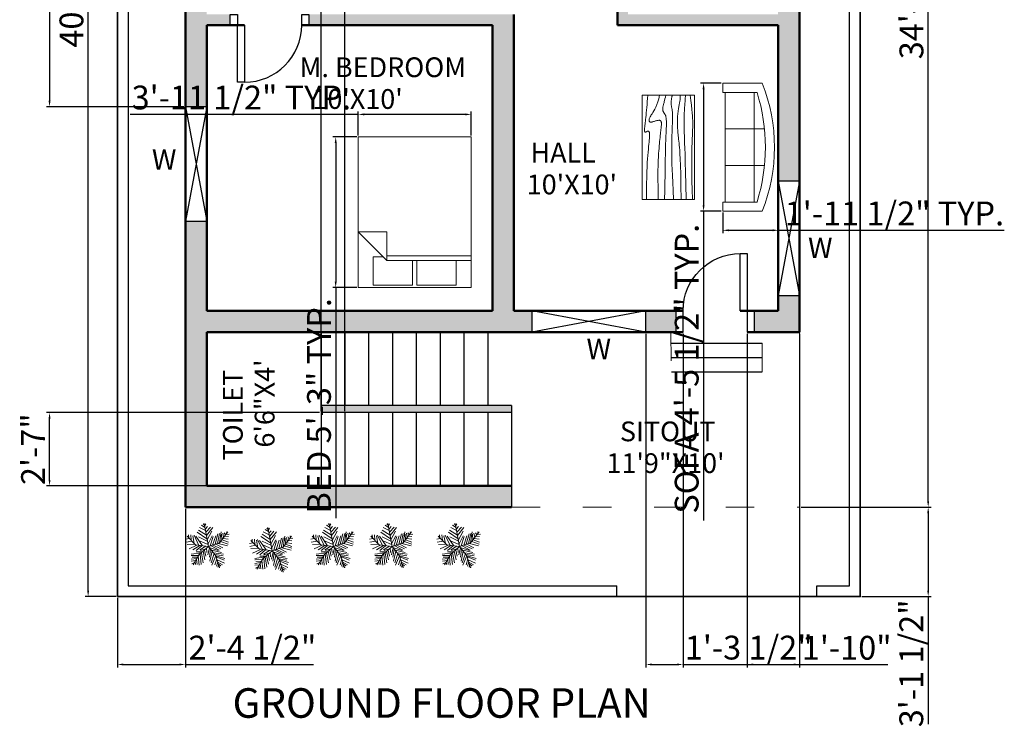
# Model space of a CAD drawing. Units: inches. Extents: x 2789 to 3623, y 2388 to 2993.
# Tile 1 of 5: x 2789 to 3203, y 2388 to 2685. Entities that reach past the tile are written whole.
import ezdxf

# ---------------------------------------------------------------- set-up
doc = ezdxf.new("R2010")
doc.units = ezdxf.units.IN
doc.linetypes.add('ACAD_ISO03W100', pattern=[30, 12, -18])
for name, color, linetype, lineweight in [('A-ANNO-DIMS', 2, 'Continuous', 18), ('A-ANNO-TEXT', 7, 'Continuous', 18), ('A-ANNO-TITL', 7, 'Continuous', 35), ('A-AREA-IDEN', 7, 'Continuous', 18), ('A-FLOR-OVHD', 8, 'ACAD_ISO03W100', 18), ('A-FLOR-STRS', 7, 'Continuous', 25), ('A-FLOR-STRS-HIDN', 7, 'ACAD_ISO03W100', 18), ('A-FURN', 8, 'Continuous', 18), ('A-WALL', 7, 'Continuous', 50), ('A-WALL-PATT', 5, 'Continuous', 13), ('C-PROP', 7, 'Continuous', 35), ('d', 1, 'Continuous', 25), ('L-PLNT', 94, 'Continuous', 13), ('L-WALL', 7, 'Continuous', 25), ('w', 170, 'Continuous', 25)]:
    doc.layers.add(name, color=color, linetype=linetype, lineweight=lineweight)
doc.styles.get("Standard").update_dxf_attribs({"font": 'arial.ttf'})
doc.dimstyles.new('ISO-25', dxfattribs={"dimtxt": 10, "dimasz": 2.5, "dimexe": 1.25, "dimexo": 0.625, "dimtad": 1, "dimlunit": 4, "dimtxsty": 'Standard', "dimcen": 2.5, "dimadec": 0, "dimazin": 0, "dimtfac": 1, "dimtmove": 0, "dimatfit": 3, "dimfxl": 1, "dimarcsym": 0})

# ---------------------------------------------------------------- blocks, each defined once
blk = doc.blocks.new('Sofa - Roundback 7 ft.')
for p, q in [((-36.000027, -34), (-36.000027, -11.4696)), ((-12.00002, -32.4421), (-12.00003, -6.5971)), ((11.99997, -32.4421), (11.99998, -6.5971)), ((35.99998, -34), (35.99998, -11.4696)), ((-35.999844, -13.3819), (35.9998, -13.3819)), ((-36.000027, -32.4421), (35.99998, -32.4421))]:
    blk.add_line(p, q)
for points in [[(-36.000027, -34), (-42.000027, -34), (-42.000027, -8)], [(41.99998, -8), (41.99998, -34), (35.99998, -34)]]:
    blk.add_lwpolyline(points)
for centre, radius, start, end in [((0, -114.25), 114.25, 68.43141, 111.5686), ((-0.00001, -127.1968), 121.1968, 72.72033, 107.2797)]:
    blk.add_arc(centre, radius, start, end)
blk = doc.blocks.new('Table - Rectangular Woodgrain 60 x 30 in.')
for p, q in [((0, 0), (0, -30)), ((60, 0), (0, 0)), ((60, -30), (60, 0)), ((0, -30), (60, -30))]:
    blk.add_line(p, q)
for points in [[(0, -2.4), (4.8155, -2.418), (9.0302, -2.4688), (12.709, -2.5477), (15.9167, -2.65), (18.7181, -2.7711), (21.1781, -2.9063), (23.3616, -3.0508), (25.3333, -3.2), (27.1477, -3.3495), (28.8172, -3.4958), (30.3437, -3.636), (31.7291, -3.7667), (32.9756, -3.8849), (34.0849, -3.9875), (35.059, -4.0714), (35.9, -4.1334), (36.6114, -4.1711), (37.2041, -4.1854), (37.6906, -4.1779), (38.0833, -4.15), (38.3948, -4.1034), (38.6375, -4.0396), (38.8239, -3.9602), (38.9666, -3.8667), (39.0764, -3.7608), (39.1573, -3.6448), (39.2116, -3.521), (39.2416, -3.3917), (39.2498, -3.2593), (39.2385, -3.1261), (39.21, -2.9944), (39.1666, -2.8667), (39.111, -2.7447), (39.0468, -2.6281), (38.978, -2.5163), (38.9083, -2.4083), (38.8418, -2.3035), (38.7823, -2.201), (38.7337, -2.1001), (38.7, -2), (38.6844, -1.9003), (38.6875, -1.8021), (38.7094, -1.707), (38.75, -1.6167), (38.8094, -1.5326), (38.8875, -1.4563), (38.9844, -1.3893), (39.1, -1.3333), (39.2351, -1.2896), (39.3937, -1.2583), (39.5804, -1.2396), (39.8, -1.2333), (40.057, -1.2396), (40.3562, -1.2583), (40.7023, -1.2896), (41.1, -1.3333), (41.5547, -1.3895), (42.0755, -1.4573), (42.6721, -1.5361), (43.3542, -1.625), (44.1316, -1.7233), (45.014, -1.8302), (46.0114, -1.9449), (47.1333, -2.0667), (48.3862, -2.1947), (49.7625, -2.3281), (51.2513, -2.4663), (52.8416, -2.6083), (54.5226, -2.7535), (56.2833, -2.9011), (58.1127, -3.0501), (60, -3.2)], [(0, -9.2), (6.5759, -9.0858), (11.9385, -9.0365), (16.2527, -9.0418), (19.6833, -9.0917), (22.3952, -9.1759), (24.5531, -9.2844), (26.322, -9.4069), (27.8666, -9.5333), (29.3241, -9.6553), (30.7203, -9.7719), (32.0532, -9.8837), (33.3208, -9.9917), (34.5213, -10.0965), (35.6526, -10.199), (36.7128, -10.2999), (37.7, -10.4), (38.6129, -10.4996), (39.4531, -10.5969), (40.223, -10.6895), (40.925, -10.775), (41.5613, -10.8512), (42.1344, -10.9156), (42.6465, -10.966), (43.1, -11), (43.4976, -11.0158), (43.8437, -11.0136), (44.143, -10.9942), (44.4, -10.9583), (44.6195, -10.9069), (44.8062, -10.8406), (44.9648, -10.7603), (45.1, -10.6667), (45.2155, -10.5598), (45.3114, -10.4365), (45.3871, -10.2929), (45.4416, -10.125), (45.4743, -9.929), (45.4844, -9.7011), (45.4709, -9.4371), (45.4333, -9.1333), (45.3716, -8.7883), (45.2896, -8.4104), (45.1919, -8.0107), (45.0833, -7.6), (44.9685, -7.1893), (44.8521, -6.7896), (44.7388, -6.4117), (44.6333, -6.0667), (44.54, -5.7628), (44.4614, -5.4979), (44.4001, -5.2675), (44.3583, -5.0667), (44.3384, -4.8909), (44.3427, -4.7354), (44.3736, -4.5956), (44.4333, -4.4667), (44.5236, -4.3453), (44.6427, -4.2333), (44.7884, -4.1339), (44.9583, -4.05), (45.1501, -3.9849), (45.3614, -3.9417), (45.59, -3.9234), (45.8333, -3.9333), (46.0915, -3.9749), (46.3734, -4.0531), (46.6906, -4.1736), (47.0542, -4.3417), (47.4756, -4.5629), (47.9661, -4.8427), (48.5372, -5.1866), (49.2, -5.6), (49.9676, -6.0844), (50.8594, -6.625), (51.8965, -7.2031), (53.1, -7.8), (54.491, -8.3969), (56.0906, -8.975), (57.9199, -9.5156), (60, -10)], [(0, -12.8), (5.1847, -12.9322), (9.6213, -13.0323), (13.3963, -13.1059), (16.5958, -13.1583), (19.3063, -13.1952), (21.614, -13.2219), (23.6054, -13.2439), (25.3666, -13.2667), (26.9728, -13.2947), (28.4531, -13.3281), (29.8256, -13.3663), (31.1083, -13.4083), (32.3191, -13.4535), (33.476, -13.501), (34.597, -13.5501), (35.7, -13.6), (36.7984, -13.6497), (37.8875, -13.6979), (38.9578, -13.743), (40, -13.7833), (41.0047, -13.8174), (41.9625, -13.8438), (42.864, -13.8607), (43.7, -13.8667), (44.4631, -13.8604), (45.1552, -13.8417), (45.7801, -13.8104), (46.3416, -13.7667), (46.8439, -13.7104), (47.2906, -13.6417), (47.6858, -13.5604), (48.0333, -13.4667), (48.3375, -13.3608), (48.6042, -13.2448), (48.8396, -13.121), (49.05, -12.9917), (49.2417, -12.8593), (49.4208, -12.7261), (49.5937, -12.5944), (49.7667, -12.4667), (49.9452, -12.3451), (50.1323, -12.2313), (50.3303, -12.1268), (50.5416, -12.0333), (50.7686, -11.9524), (51.0135, -11.8854), (51.2788, -11.8341), (51.5666, -11.8), (51.8785, -11.7843), (52.2116, -11.7865), (52.562, -11.8059), (52.926, -11.8417), (53.2998, -11.8931), (53.6795, -11.9594), (54.0614, -12.0397), (54.4416, -12.1333), (54.8223, -12.2401), (55.2293, -12.3625), (55.6942, -12.5037), (56.2489, -12.6667), (56.9251, -12.8547), (57.7545, -13.0708), (58.7689, -13.3182), (60, -13.6)], [(0, -18), (5.124, -17.7273), (9.6609, -17.5057), (13.6705, -17.3303), (17.2125, -17.1958), (20.3467, -17.0973), (23.1328, -17.0297), (25.6307, -16.9878), (27.9, -16.9667), (29.9928, -16.9617), (31.9302, -16.9703), (33.7254, -16.9907), (35.3917, -17.0208), (36.9423, -17.0588), (38.3906, -17.1026), (39.7499, -17.1503), (41.0333, -17.2), (42.2519, -17.2496), (43.4073, -17.2969), (44.4986, -17.3395), (45.525, -17.375), (46.4858, -17.4012), (47.3802, -17.4156), (48.2074, -17.416), (48.9667, -17.4), (49.6583, -17.3662), (50.2872, -17.3167), (50.8595, -17.2547), (51.3812, -17.1833), (51.8584, -17.1057), (52.2971, -17.025), (52.7034, -16.9443), (53.0833, -16.8667), (53.443, -16.7951), (53.789, -16.7313), (54.128, -16.6768), (54.4666, -16.6334), (54.8115, -16.6024), (55.1693, -16.5854), (55.5465, -16.5841), (55.95, -16.6), (56.3828, -16.6337), (56.8346, -16.6823), (57.2915, -16.7418), (57.7396, -16.8084), (58.165, -16.878), (58.5539, -16.9469), (58.8924, -17.0111), (59.1666, -17.0667), (59.3679, -17.1107), (59.5078, -17.1438), (59.6032, -17.1675), (59.6708, -17.1833), (59.7275, -17.193), (59.7901, -17.1979), (59.8753, -17.1998), (60, -17.2)], [(0, -22.4), (8.0098, -22.2501), (14.4094, -22.1011), (19.4168, -21.9535), (23.25, -21.8083), (26.1269, -21.6663), (28.2656, -21.5281), (29.884, -21.3947), (31.2, -21.2667), (32.3967, -21.1448), (33.5172, -21.0292), (34.5697, -20.9198), (35.5625, -20.8167), (36.5037, -20.7198), (37.4015, -20.6292), (38.2642, -20.5448), (39.1, -20.4667), (39.9164, -20.3951), (40.7187, -20.3313), (41.5117, -20.2768), (42.3, -20.2333), (43.0883, -20.2024), (43.8812, -20.1854), (44.6836, -20.1841), (45.5, -20.2), (46.3328, -20.234), (47.1747, -20.2844), (48.0163, -20.3488), (48.8479, -20.425), (49.66, -20.5106), (50.4429, -20.6031), (51.1872, -20.7004), (51.8833, -20.8), (52.5246, -20.8999), (53.1166, -20.9995), (53.6681, -21.0983), (54.1875, -21.1958), (54.6834, -21.2919), (55.1646, -21.3859), (55.6394, -21.4777), (56.1167, -21.5667), (56.6028, -21.6515), (57.0961, -21.7266), (57.5929, -21.7852), (58.0896, -21.8208), (58.5823, -21.8268), (59.0674, -21.7964), (59.5412, -21.723), (60, -21.6)], [(0, -25.2), (8.6355, -25.0504), (15.7026, -24.9031), (21.4049, -24.7606), (25.9458, -24.625), (29.529, -24.4988), (32.3578, -24.3844), (34.6359, -24.284), (36.5667, -24.2), (38.3213, -24.1341), (39.9417, -24.0854), (41.437, -24.0523), (42.8167, -24.0333), (44.0901, -24.0268), (45.2667, -24.0313), (46.3557, -24.0451), (47.3667, -24.0667), (48.309, -24.0947), (49.1928, -24.1287), (50.0284, -24.168), (50.826, -24.2125), (51.5959, -24.2617), (52.3483, -24.3151), (53.0935, -24.3725), (53.8417, -24.4334), (54.6009, -24.497), (55.3699, -24.561), (56.1454, -24.6226), (56.9239, -24.6792), (57.7021, -24.7279), (58.4764, -24.7662), (59.2435, -24.7911), (60, -24.8)], [(0, -28.8), (5.6867, -28.6681), (10.45, -28.5698), (14.407, -28.5012), (17.675, -28.4584), (20.3711, -28.4374), (22.6125, -28.4344), (24.5164, -28.4455), (26.2, -28.4667), (27.762, -28.4947), (29.2276, -28.5281), (30.6033, -28.5663), (31.8958, -28.6084), (33.1118, -28.6535), (34.2578, -28.7011), (35.3405, -28.7501), (36.3666, -28.8), (37.3443, -28.8497), (38.288, -28.8974), (39.2137, -28.9412), (40.1375, -28.9792), (41.0753, -29.0093), (42.0432, -29.0297), (43.0572, -29.0384), (44.1333, -29.0333), (45.2936, -29.0114), (46.5843, -28.9641), (48.0579, -28.8816), (49.7666, -28.7542), (51.7629, -28.5721), (54.0989, -28.3255), (56.8272, -28.0048), (60, -27.6)]]:
    blk.add_lwpolyline(points)
blk = doc.blocks.new('Bed - Queen')
for p, q in [((0, -80.00003), (0, 0)), ((0, 0), (59.99999, 0)), ((59.99999, 0), (59.99999, -80.00003)), ((7.99999, -1.2), (28.79998, -1.2)), ((7.99999, -14.4), (7.99999, -1.2)), ((28.79998, -1.2), (28.79998, -14.4)), ((31.19999, -1.2), (51.99999, -1.2)), ((31.19999, -14.4), (31.19999, -1.2)), ((51.99999, -1.2), (51.99999, -16.4)), ((0, -14.4), (44.8, -14.4)), ((59.99999, -29.6), (44.8, -14.4)), ((44.8, -14.4), (44.8, -29.6)), ((44.8, -16.8), (0, -16.8)), ((51.99999, -16.4), (46.79936, -16.4)), ((44.8, -29.6), (59.99999, -29.6)), ((59.99999, -80.00003), (0, -80.00003))]:
    blk.add_line(p, q)
blk = doc.blocks.new('*U11')
for p, q in [((-8.737, 47.138), (-17.069, 52.711)), ((-10.186, 53.64), (-13.084, 55.962)), ((0, 0), (-10.5, 57)), ((-9.099, 51.782), (-6.563, 55.962)), ((-7.65, 43.423), (-2.578, 49.46)), ((-31.5, 4.5), (-52.5, 25.5)), ((-48.585, 21.131), (-49.309, 29.026)), ((-43.513, 28.561), (-42.427, 15.558)), ((-38.442, 26.239), (-34.819, 7.663)), ((-35.544, 28.097), (-24.314, 3.947)), ((-14.533, 2.09), (-30.834, 25.31)), ((-3.665, 19.273), (-27.574, 35.527)), ((-5.114, 28.097), (-24.676, 40.636)), ((-7.288, 39.707), (-21.778, 46.673)), ((-5.839, 35.992), (4.667, 48.067)), ((-5.114, 27.632), (10.463, 46.673)), ((-2.941, 16.486), (8.652, 37.85)), ((-1.129, 6.734), (9.014, 26.704)), ((3.942, 1.625), (11.187, 24.381)), ((10.101, 3.483), (17.708, 26.239)), ((16.259, 5.805), (23.142, 31.348)), ((22.055, 7.198), (27.489, 32.277)), ((27, 9), (48, 36)), ((27.127, 9.056), (31.112, 35.992)), ((31.836, 30.883), (32.561, 16.486)), ((35.096, 32.741), (37.27, 22.524)), ((38.719, 34.134), (41.979, 28.561)), ((40.53, 25.775), (48.862, 24.846)), ((43.791, 29.954), (51.036, 30.883)), ((44.153, 36.456), (45.239, 32.741)), ((-47.498, 19.737), (-55.83, 18.344)), ((-40.615, 13.7), (-55.105, 10.913)), ((-33.37, 6.269), (-52.207, 5.34)), ((-28.299, 3.483), (-47.86, -5.805)), ((-21.416, 3.018), (-38.079, -8.128)), ((0, 0), (-31.5, 4.5)), ((-15.982, 2.09), (-30.11, -9.521)), ((-24.314, 23.917), (-2.941, 13.7)), ((0, 0), (-22.5, -19.5)), ((-6.563, 1.161), (-21.416, -8.128)), ((-20.691, 13.7), (-1.129, 4.876)), ((0, 0), (27, 9)), ((0, 0), (18, -22.5)), ((6.478, 1.625), (26.04, -8.592)), ((11.187, 3.483), (30.749, -5.805)), ((18.07, 5.805), (35.096, -3.483)), ((24.229, 7.663), (46.688, 1.625)), ((29.662, 12.307), (48.137, 6.269)), ((33.285, 16.486), (48.862, 10.913)), ((36.183, 19.737), (48.137, 17.88)), ((-17.431, -15.094), (-42.789, -18.809)), ((-24.314, -21.596), (-42.427, -22.06)), ((-22.5, -19.5), (-37.5, -45)), ((-15.257, -12.772), (-30.11, -12.772)), ((-25.038, -23.918), (-22.865, -45.281)), ((-20.691, -18.345), (-17.793, -44.352)), ((-6.563, -5.805), (-19.967, -9.985)), ((-17.069, -15.094), (-12.721, -40.172)), ((-13.446, -11.378), (-8.737, -32.741)), ((-9.461, -8.592), (-6.201, -23.453)), ((-4.752, -3.483), (-3.665, -14.629)), ((2.493, -3.019), (-1.491, -20.202)), ((1.769, -2.555), (24.229, -9.521)), ((5.029, -6.27), (2.131, -25.775)), ((9.014, -11.378), (3.58, -35.992)), ((14.085, -16.951), (6.478, -40.172)), ((7.565, -9.056), (32.198, -14.629)), ((18.07, -22.524), (8.289, -45.745)), ((12.274, -15.094), (36.907, -18.809)), ((16.259, -19.738), (36.183, -22.989)), ((18, -22.5), (27, -52.5)), ((18.433, -22.524), (40.53, -29.026)), ((-28.299, -29.026), (-42.789, -31.348)), ((-30.834, -34.135), (-42.427, -35.528)), ((-34.457, -39.708), (-40.978, -42.494)), ((-26.849, -26.24), (-40.253, -25.775)), ((-32.646, -36.921), (-31.921, -44.352)), ((-29.023, -30.884), (-27.936, -43.887)), ((20.244, -30.419), (15.897, -44.816)), ((19.157, -25.311), (38.719, -33.206)), ((22.78, -37.85), (19.519, -48.532)), ((21.331, -32.741), (39.081, -40.636)), ((22.78, -38.314), (34.372, -44.816)), ((24.591, -45.745), (23.142, -50.854)), ((24.591, -43.423), (30.749, -47.603)), ((26.764, -49.925), (28.213, -50.854))]:
    blk.add_line(p, q)
blk = doc.blocks.new('*D13')
at = {"layer": 'A-ANNO-DIMS', "color": 0, "lineweight": -2, "transparency": 16777216}
for p, q in [((2829.92, 2922.84), (2816.96, 2922.84)), ((2818.21, 2445.34), (2818.21, 2920.34)), ((2829.92, 2442.84), (2816.96, 2442.84))]:
    blk.add_line(p, q, dxfattribs=at)
at = {"layer": 'A-ANNO-DIMS', "color": 0, "transparency": 16777216}
for points in [[(2817.8, 2920.34), (2818.63, 2920.34), (2818.21, 2922.84)], [(2817.8, 2445.34), (2818.63, 2445.34), (2818.21, 2442.84)]]:
    blk.add_solid(points, dxfattribs=at)
at = {"layer": 'Defpoints', "color": 0, "transparency": 16777216}
for p in [(2818.21, 2922.84), (2830.55, 2922.84), (2830.55, 2442.84)]:
    blk.add_point(p, dxfattribs=at)
at = {"layer": 'A-ANNO-DIMS', "color": 0, "transparency": 16777216, "insert": (2812.48, 2682.84), "char_height": 10, "attachment_point": 5, "rotation": 90}
blk.add_mtext("40'", dxfattribs=at)
blk = doc.blocks.new('DOOR-24IN-JAMB-9IN')
for points in [[(0, 24), (-3, 24), (-3, 0), (0, 0)], [(-6, 0), (-3, 0), (-3, -9), (-6, -9)], [(24, 0), (27, 0), (27, -9), (24, -9)]]:
    blk.add_lwpolyline(points, close=True)
blk.add_arc((0, 0), 24, 0, 90)
blk = doc.blocks.new('DOOR-24IN-JAMB-4_5IN')
for points in [[(-3, 0), (-6, 0), (-6, 4.5), (-3, 4.5)], [(27, 0), (24, 0), (24, 4.5), (27, 4.5)], [(0, -24), (-3, -24), (-3, 0), (0, 0)]]:
    blk.add_lwpolyline(points, close=True)
blk.add_arc((0, 0), 24, 270, 0)
blk = doc.blocks.new('WINDOW-48IN')
for p, q in [((48, 9), (0, 0)), ((48, 0), (0, 9))]:
    blk.add_line(p, q)
blk.add_lwpolyline([(0, 9), (0, 0), (48, 0), (48, 9)], close=True)
blk = doc.blocks.new('*D26')
at = {"layer": 'A-ANNO-DIMS', "color": 0, "lineweight": -2, "transparency": 16777216}
for p, q in [((2931.06, 2635.83), (2920.95, 2635.83)), ((2922.2, 2633.33), (2922.2, 2575.1)), ((2931.06, 2572.6), (2920.95, 2572.6)), ((2922.2, 2572.6), (2922.2, 2475.74))]:
    blk.add_line(p, q, dxfattribs=at)
at = {"layer": 'A-ANNO-DIMS', "color": 0, "transparency": 16777216}
for points in [[(2921.79, 2633.33), (2922.62, 2633.33), (2922.2, 2635.83)], [(2921.79, 2575.1), (2922.62, 2575.1), (2922.2, 2572.6)]]:
    blk.add_solid(points, dxfattribs=at)
at = {"layer": 'Defpoints', "color": 0, "transparency": 16777216}
for p in [(2931.69, 2635.83), (2922.2, 2572.6), (2931.69, 2572.6)]:
    blk.add_point(p, dxfattribs=at)
at = {"layer": 'A-ANNO-DIMS', "color": 0, "transparency": 16777216, "insert": (2916.47, 2522.92), "char_height": 10, "attachment_point": 5, "rotation": 90}
blk.add_mtext('BED 5\'-3" TYP.', dxfattribs=at)
blk = doc.blocks.new('*D27')
at = {"layer": 'A-ANNO-DIMS', "color": 0, "lineweight": -2, "transparency": 16777216}
for p, q in [((2931.69, 2645.31), (2835.92, 2645.31)), ((2931.69, 2636.45), (2931.69, 2646.56)), ((2976.61, 2645.31), (2934.19, 2645.31)), ((2979.11, 2636.45), (2979.11, 2646.56))]:
    blk.add_line(p, q, dxfattribs=at)
at = {"layer": 'A-ANNO-DIMS', "color": 0, "transparency": 16777216}
for points in [[(2934.19, 2645.73), (2934.19, 2644.9), (2931.69, 2645.31)], [(2976.61, 2645.73), (2976.61, 2644.9), (2979.11, 2645.31)]]:
    blk.add_solid(points, dxfattribs=at)
at = {"layer": 'Defpoints', "color": 0, "transparency": 16777216}
for p in [(2931.69, 2645.31), (2931.69, 2635.83), (2979.11, 2635.83)]:
    blk.add_point(p, dxfattribs=at)
at = {"layer": 'A-ANNO-DIMS', "color": 0, "transparency": 16777216, "insert": (2882.55, 2651.11), "char_height": 10, "attachment_point": 5}
blk.add_mtext('3\'-11 1/2" TYP.', dxfattribs=at)
blk = doc.blocks.new('*D32')
at = {"layer": 'A-ANNO-DIMS', "color": 0, "lineweight": -2, "transparency": 16777216}
for p, q in [((3084.17, 2658.4), (3075.49, 2658.4)), ((3076.74, 2655.9), (3076.74, 2607.19)), ((3084.17, 2604.69), (3075.49, 2604.69)), ((3076.74, 2604.69), (3076.74, 2474.82))]:
    blk.add_line(p, q, dxfattribs=at)
at = {"layer": 'A-ANNO-DIMS', "color": 0, "transparency": 16777216}
for points in [[(3076.33, 2655.9), (3077.16, 2655.9), (3076.74, 2658.4)], [(3076.33, 2607.19), (3077.16, 2607.19), (3076.74, 2604.69)]]:
    blk.add_solid(points, dxfattribs=at)
at = {"layer": 'Defpoints', "color": 0, "transparency": 16777216}
for p in [(3084.8, 2658.4), (3076.74, 2604.69), (3084.8, 2604.69)]:
    blk.add_point(p, dxfattribs=at)
at = {"layer": 'A-ANNO-DIMS', "color": 0, "transparency": 16777216, "insert": (3070.94, 2538.5), "char_height": 10, "attachment_point": 5, "rotation": 90}
blk.add_mtext('SOFA 4\'-5 1/2" TYP.', dxfattribs=at)
blk = doc.blocks.new('*D33')
at = {"layer": 'A-ANNO-DIMS', "color": 0, "lineweight": -2, "transparency": 16777216}
for p, q in [((3084.8, 2604.07), (3084.8, 2595.38)), ((3108.24, 2604.07), (3108.24, 2595.38)), ((3087.3, 2596.63), (3105.74, 2596.63)), ((3108.24, 2596.63), (3203.08, 2596.63))]:
    blk.add_line(p, q, dxfattribs=at)
at = {"layer": 'A-ANNO-DIMS', "color": 0, "transparency": 16777216}
for points in [[(3087.3, 2597.05), (3087.3, 2596.22), (3084.8, 2596.63)], [(3105.74, 2597.05), (3105.74, 2596.22), (3108.24, 2596.63)]]:
    blk.add_solid(points, dxfattribs=at)
at = {"layer": 'Defpoints', "color": 0, "transparency": 16777216}
for p in [(3084.8, 2604.69), (3108.24, 2604.69), (3108.24, 2596.63)]:
    blk.add_point(p, dxfattribs=at)
at = {"layer": 'A-ANNO-DIMS', "color": 0, "transparency": 16777216, "insert": (3156.91, 2602.43), "char_height": 10, "attachment_point": 5}
blk.add_mtext('1\'-11 1/2" TYP.', dxfattribs=at)
blk = doc.blocks.new('*D43')
at = {"layer": 'A-ANNO-DIMS', "color": 0, "lineweight": -2, "transparency": 16777216}
for p, q in [((3117.67, 2894.34), (3172.35, 2894.34)), ((3171.1, 2482.84), (3171.1, 2891.84)), ((3117.67, 2480.34), (3172.35, 2480.34))]:
    blk.add_line(p, q, dxfattribs=at)
at = {"layer": 'A-ANNO-DIMS', "color": 0, "transparency": 16777216}
for points in [[(3170.68, 2891.84), (3171.51, 2891.84), (3171.1, 2894.34)], [(3170.68, 2482.84), (3171.51, 2482.84), (3171.1, 2480.34)]]:
    blk.add_solid(points, dxfattribs=at)
at = {"layer": 'Defpoints', "color": 0, "transparency": 16777216}
for p in [(3117.05, 2894.34), (3171.1, 2894.34), (3117.05, 2480.34)]:
    blk.add_point(p, dxfattribs=at)
at = {"layer": 'A-ANNO-DIMS', "color": 0, "transparency": 16777216, "insert": (3165.36, 2687.34), "char_height": 10, "attachment_point": 5, "rotation": 90}
blk.add_mtext('34\'-6"', dxfattribs=at)
blk = doc.blocks.new('*D46')
at = {"layer": 'A-ANNO-DIMS', "color": 0, "lineweight": -2, "transparency": 16777216}
for p, q in [((2859.05, 2479.72), (2859.05, 2413.04)), ((2830.55, 2442.22), (2830.55, 2413.04)), ((2833.05, 2414.29), (2856.55, 2414.29)), ((2859.05, 2414.29), (2912.85, 2414.29))]:
    blk.add_line(p, q, dxfattribs=at)
at = {"layer": 'A-ANNO-DIMS', "color": 0, "transparency": 16777216}
for points in [[(2833.05, 2414.71), (2833.05, 2413.88), (2830.55, 2414.29)], [(2856.55, 2414.71), (2856.55, 2413.88), (2859.05, 2414.29)]]:
    blk.add_solid(points, dxfattribs=at)
at = {"layer": 'Defpoints', "color": 0, "transparency": 16777216}
for p in [(2859.05, 2480.34), (2830.55, 2442.84), (2859.05, 2414.29)]:
    blk.add_point(p, dxfattribs=at)
at = {"layer": 'A-ANNO-DIMS', "color": 0, "transparency": 16777216, "insert": (2887.2, 2420.09), "char_height": 10, "attachment_point": 5}
blk.add_mtext('2\'-4 1/2"', dxfattribs=at)
blk = doc.blocks.new('*D47')
at = {"layer": 'A-ANNO-DIMS', "color": 0, "lineweight": -2, "transparency": 16777216}
for p, q in [((3117.67, 2480.34), (3172.35, 2480.34)), ((3171.1, 2477.84), (3171.1, 2445.34)), ((3143.17, 2442.84), (3172.35, 2442.84)), ((3171.1, 2442.84), (3171.1, 2389.21))]:
    blk.add_line(p, q, dxfattribs=at)
at = {"layer": 'A-ANNO-DIMS', "color": 0, "transparency": 16777216}
for points in [[(3170.68, 2477.84), (3171.51, 2477.84), (3171.1, 2480.34)], [(3170.68, 2445.34), (3171.51, 2445.34), (3171.1, 2442.84)]]:
    blk.add_solid(points, dxfattribs=at)
at = {"layer": 'Defpoints', "color": 0, "transparency": 16777216}
for p in [(3117.05, 2480.34), (3142.55, 2442.84), (3171.1, 2442.84)]:
    blk.add_point(p, dxfattribs=at)
at = {"layer": 'A-ANNO-DIMS', "color": 0, "transparency": 16777216, "insert": (3165.3, 2414.78), "char_height": 10, "attachment_point": 5, "rotation": 90}
blk.add_mtext('3\'-1 1/2"', dxfattribs=at)
blk = doc.blocks.new('*D48')
at = {"layer": 'A-ANNO-DIMS', "color": 0, "lineweight": -2, "transparency": 16777216}
for p, q in [((2916.05, 2520.72), (2916.05, 2952.64)), ((2918.55, 2951.39), (2923.55, 2951.39)), ((2926.05, 2520.72), (2926.05, 2952.64)), ((2926.05, 2951.39), (2964.15, 2951.39))]:
    blk.add_line(p, q, dxfattribs=at)
at = {"layer": 'A-ANNO-DIMS', "color": 0, "transparency": 16777216}
for points in [[(2918.55, 2951.81), (2918.55, 2950.98), (2916.05, 2951.39)], [(2923.55, 2951.81), (2923.55, 2950.98), (2926.05, 2951.39)]]:
    blk.add_solid(points, dxfattribs=at)
at = {"layer": 'Defpoints', "color": 0, "transparency": 16777216}
for p in [(2926.05, 2951.39), (2916.05, 2520.09), (2926.05, 2520.09)]:
    blk.add_point(p, dxfattribs=at)
at = {"layer": 'A-ANNO-DIMS', "color": 0, "transparency": 16777216, "insert": (2946.35, 2957.12), "char_height": 10, "attachment_point": 5}
blk.add_mtext('0\'-10"', dxfattribs=at)
blk = doc.blocks.new('*D49')
at = {"layer": 'A-ANNO-DIMS', "color": 0, "lineweight": -2, "transparency": 16777216}
for p, q in [((2915.42, 2520.09), (2800.75, 2520.09)), ((2802, 2491.84), (2802, 2517.59)), ((2915.42, 2489.34), (2800.75, 2489.34))]:
    blk.add_line(p, q, dxfattribs=at)
at = {"layer": 'A-ANNO-DIMS', "color": 0, "transparency": 16777216}
for points in [[(2801.58, 2517.59), (2802.41, 2517.59), (2802, 2520.09)], [(2801.58, 2491.84), (2802.41, 2491.84), (2802, 2489.34)]]:
    blk.add_solid(points, dxfattribs=at)
at = {"layer": 'Defpoints', "color": 0, "transparency": 16777216}
for p in [(2802, 2520.09), (2916.05, 2520.09), (2916.05, 2489.34)]:
    blk.add_point(p, dxfattribs=at)
at = {"layer": 'A-ANNO-DIMS', "color": 0, "transparency": 16777216, "insert": (2796.35, 2504.72), "char_height": 10, "attachment_point": 5, "rotation": 90}
blk.add_mtext('2\'-7"', dxfattribs=at)
blk = doc.blocks.new('*D53')
at = {"layer": 'A-ANNO-DIMS', "color": 0, "lineweight": -2, "transparency": 16777216}
for p, q in [((2858.42, 2771.27), (2800.75, 2771.27)), ((2802, 2768.77), (2802, 2651.02)), ((2858.42, 2648.52), (2800.75, 2648.52))]:
    blk.add_line(p, q, dxfattribs=at)
at = {"layer": 'A-ANNO-DIMS', "color": 0, "transparency": 16777216}
for points in [[(2801.58, 2768.77), (2802.41, 2768.77), (2802, 2771.27)], [(2801.58, 2651.02), (2802.41, 2651.02), (2802, 2648.52)]]:
    blk.add_solid(points, dxfattribs=at)
at = {"layer": 'Defpoints', "color": 0, "transparency": 16777216}
for p in [(2859.05, 2771.27), (2802, 2648.52), (2859.05, 2648.52)]:
    blk.add_point(p, dxfattribs=at)
at = {"layer": 'A-ANNO-DIMS', "color": 0, "transparency": 16777216, "insert": (2796.26, 2709.89), "char_height": 10, "attachment_point": 5, "rotation": 90}
blk.add_mtext('10\'-3"', dxfattribs=at)
blk = doc.blocks.new('*D57')
at = {"layer": 'A-ANNO-DIMS', "color": 0, "lineweight": -2, "transparency": 16777216}
for p, q in [((3052.55, 2553.22), (3052.55, 2413.04)), ((3068.12, 2553.22), (3068.12, 2413.04)), ((3055.05, 2414.29), (3065.62, 2414.29)), ((3068.12, 2414.29), (3120.81, 2414.29))]:
    blk.add_line(p, q, dxfattribs=at)
at = {"layer": 'A-ANNO-DIMS', "color": 0, "transparency": 16777216}
for points in [[(3055.05, 2414.71), (3055.05, 2413.88), (3052.55, 2414.29)], [(3065.62, 2414.71), (3065.62, 2413.88), (3068.12, 2414.29)]]:
    blk.add_solid(points, dxfattribs=at)
at = {"layer": 'Defpoints', "color": 0, "transparency": 16777216}
for p in [(3052.55, 2553.84), (3068.12, 2553.84), (3068.12, 2414.29)]:
    blk.add_point(p, dxfattribs=at)
at = {"layer": 'A-ANNO-DIMS', "color": 0, "transparency": 16777216, "insert": (3095.71, 2420.09), "char_height": 10, "attachment_point": 5}
blk.add_mtext('1\'-3 1/2"', dxfattribs=at)
blk = doc.blocks.new('*D58')
at = {"layer": 'A-ANNO-DIMS', "color": 0, "lineweight": -2, "transparency": 16777216}
for p, q in [((3095.12, 2553.22), (3095.12, 2413.04)), ((3117.05, 2553.22), (3117.05, 2413.04)), ((3097.62, 2414.29), (3114.55, 2414.29)), ((3117.05, 2414.29), (3154.21, 2414.29))]:
    blk.add_line(p, q, dxfattribs=at)
at = {"layer": 'A-ANNO-DIMS', "color": 0, "transparency": 16777216}
for points in [[(3097.62, 2414.71), (3097.62, 2413.88), (3095.12, 2414.29)], [(3114.55, 2414.71), (3114.55, 2413.88), (3117.05, 2414.29)]]:
    blk.add_solid(points, dxfattribs=at)
at = {"layer": 'Defpoints', "color": 0, "transparency": 16777216}
for p in [(3095.12, 2553.84), (3117.05, 2553.84), (3117.05, 2414.29)]:
    blk.add_point(p, dxfattribs=at)
at = {"layer": 'A-ANNO-DIMS', "color": 0, "transparency": 16777216, "insert": (3136.88, 2420.02), "char_height": 10, "attachment_point": 5}
blk.add_mtext('1\'-10"', dxfattribs=at)

msp = doc.modelspace()

# ---------------------------------------------------------------- hatches: boundary and pattern name
at = {"layer": 'A-WALL-PATT'}
h = msp.add_hatch(color=256, dxfattribs=at)
h.dxf.hatch_style = 1
h.paths.add_polyline_path([(2868.048, 2600.516), (2859.048, 2600.516), (2859.048, 2480.342), (2996.048, 2480.342), (2996.048, 2489.342), (2868.048, 2489.342), (2868.048, 2553.842), (3004.548, 2553.842), (3004.548, 2562.842), (2997.048, 2562.842), (2997.048, 2687.342), (2910.917, 2687.342), (2910.917, 2682.842), (2988.048, 2682.842), (2988.048, 2562.842), (2868.048, 2562.842)])
h.paths.add_polyline_path([(2996.048, 2523.092), (2916.048, 2523.092), (2916.048, 2520.092), (2996.048, 2520.092)], flags=17)
h.paths.add_polyline_path([(3065.118, 2562.842), (3052.548, 2562.842), (3052.548, 2553.842), (3065.118, 2553.842)])
h.paths.add_polyline_path([(3117.048, 2569.319), (3108.048, 2569.319), (3108.048, 2562.842), (3098.118, 2562.842), (3098.118, 2553.842), (3117.048, 2553.842)])
h.paths.add_polyline_path([(3117.048, 2707.71), (3108.048, 2707.71), (3108.048, 2687.342), (3045.048, 2687.342), (3045.048, 2756.342), (3057.181, 2756.342), (3057.181, 2765.342), (3034.539, 2765.342), (3034.539, 2756.342), (3040.548, 2756.342), (3040.548, 2682.842), (3108.048, 2682.842), (3108.048, 2617.319), (3117.048, 2617.319)])
h.paths.add_polyline_path([(3117.048, 2817.229), (3108.048, 2817.229), (3108.048, 2812.239), (3108.048, 2765.342), (3090.181, 2765.342), (3090.181, 2756.342), (3108.048, 2756.342), (3108.048, 2731.71), (3117.048, 2731.71)])
h.paths.add_polyline_path([(2868.048, 2682.842), (2877.917, 2682.842), (2877.917, 2687.342), (2868.048, 2687.342), (2868.048, 2756.342), (2889.977, 2756.342), (2889.977, 2765.342), (2868.048, 2765.342), (2868.048, 2771.267), (2859.048, 2771.267), (2859.048, 2648.516), (2868.048, 2648.516)])
h.paths.add_polyline_path([(3001.539, 2765.342), (2997.048, 2765.342), (2997.048, 2885.342), (3001.182, 2885.342), (3001.182, 2894.342), (2920.184, 2894.342), (2920.184, 2885.342), (2988.048, 2885.342), (2988.048, 2765.342), (2925.977, 2765.342), (2925.977, 2756.342), (3001.539, 2756.342)])
h.paths.add_polyline_path([(2868.048, 2885.342), (2872.184, 2885.342), (2872.184, 2894.342), (2859.048, 2894.342), (2859.048, 2819.267), (2868.048, 2819.267)])
h.paths.add_polyline_path([(3117.048, 2894.342), (3049.182, 2894.342), (3049.182, 2885.342), (3108.048, 2885.342), (3108.048, 2865.229), (3117.048, 2865.229)])
h.paths.add_polyline_path([(3025.421, 2540.366), (3041.067, 2540.366), (3041.067, 2553.271), (3025.421, 2553.271)], flags=9)
h.paths.add_polyline_path([(3118.771, 2839.078), (3134.416, 2839.078), (3134.416, 2851.983), (3118.771, 2851.983)], flags=9)
h.paths.add_polyline_path([(3118.682, 2712.44), (3131, 2712.44), (3131, 2725.345), (3118.682, 2725.345)], flags=9)
h.paths.add_polyline_path([(3118.47, 2582.859), (3134.115, 2582.859), (3134.115, 2595.763), (3118.47, 2595.763)], flags=9)
h.paths.add_polyline_path([(2842.843, 2619.924), (2858.489, 2619.924), (2858.489, 2632.829), (2842.843, 2632.829)], flags=9)
h.paths.add_polyline_path([(2841.723, 2794.475), (2857.368, 2794.475), (2857.368, 2807.38), (2841.723, 2807.38)], flags=9)
h.paths.add_polyline_path([(3018.872, 2895.803), (3034.517, 2895.803), (3034.517, 2908.708), (3018.872, 2908.708)], flags=9)
h.paths.add_polyline_path([(2891.065, 2897.701), (2906.71, 2897.701), (2906.71, 2910.606), (2891.065, 2910.606)], flags=9)
h.paths.add_polyline_path([(2898.76, 2503.274), (2898.76, 2543.14), (2886.045, 2543.14), (2886.045, 2503.274)], flags=25)
h.paths.add_polyline_path([(2885.453, 2497.829), (2885.453, 2542.718), (2872.568, 2542.718), (2872.568, 2497.829)], flags=25)
h.paths.add_polyline_path([(3033.853, 2492.441), (3086.618, 2492.441), (3086.618, 2505.156), (3033.853, 2505.156)], flags=9)
h.paths.add_polyline_path([(3039.46, 2505.748), (3086.274, 2505.748), (3086.274, 2518.633), (3039.46, 2518.633)], flags=9)
h.paths.add_polyline_path([(3048.345, 2778.023), (3090.544, 2778.023), (3090.544, 2790.738), (3048.345, 2790.738)], flags=9)
h.paths.add_polyline_path([(3024.618, 2791.33), (3106.873, 2791.33), (3106.873, 2804.214), (3024.618, 2804.214)], flags=9)
h.paths.add_polyline_path([(3047.007, 2712.567), (3076.988, 2712.567), (3076.988, 2720.13), (3047.007, 2720.13)], flags=25)
h.paths.add_polyline_path([(3050.563, 2720.481), (3079.162, 2720.481), (3079.162, 2728.14), (3050.563, 2728.14)], flags=25)
h.paths.add_polyline_path([(3000.345, 2609.496), (3042.544, 2609.496), (3042.544, 2622.211), (3000.345, 2622.211)], flags=9)
h.paths.add_polyline_path([(3001.972, 2623.016), (3035.131, 2623.016), (3035.131, 2635.468), (3001.972, 2635.468)], flags=9)
h.paths.add_polyline_path([(2910.315, 2645.374), (2952.514, 2645.374), (2952.514, 2658.089), (2910.315, 2658.089)], flags=25)
h.paths.add_polyline_path([(2904.87, 2658.68), (2985.189, 2658.68), (2985.189, 2671.565), (2904.87, 2671.565)], flags=25)
h.paths.add_polyline_path([(2902.494, 2717.778), (2948.81, 2717.778), (2948.81, 2730.493), (2902.494, 2730.493)], flags=9)
h.paths.add_polyline_path([(2897.051, 2731.086), (2956.772, 2731.086), (2956.772, 2743.962), (2897.051, 2743.962)], flags=9)
h.paths.add_polyline_path([(2902.494, 2806.621), (2944.693, 2806.621), (2944.693, 2819.336), (2902.494, 2819.336)], flags=9)
h.paths.add_polyline_path([(2897.051, 2819.929), (2955.464, 2819.929), (2955.464, 2832.806), (2897.051, 2832.806)], flags=9)

# ---------------------------------------------------------------- linework, layer by layer
at = {"layer": 'A-FLOR-OVHD'}
for p in [(3117.048, 2553.842), (2996.048, 2480.342)]:
    msp.add_line(p, (3117.048, 2480.342), dxfattribs=at)
at = {"layer": 'A-FLOR-STRS'}
for p, q in [((2916.048, 2553.842), (2916.048, 2489.342)), ((2926.048, 2553.842), (2926.048, 2523.092)), ((2936.048, 2553.842), (2936.048, 2523.092)), ((2946.048, 2553.842), (2946.048, 2523.092)), ((2956.048, 2553.842), (2956.048, 2523.092)), ((2966.048, 2553.842), (2966.048, 2523.092)), ((2976.048, 2553.842), (2976.048, 2523.092)), ((2986.048, 2553.842), (2986.048, 2523.092)), ((3063.257, 2549.179), (3101.368, 2549.179)), ((3063.257, 2543.179), (3101.368, 2543.179)), ((3063.257, 2537.179), (3101.368, 2537.179)), ((2996.048, 2523.092), (2916.048, 2523.092)), ((2996.048, 2520.092), (2916.048, 2520.092)), ((2926.048, 2520.092), (2926.048, 2489.342)), ((2936.048, 2520.092), (2936.048, 2489.342)), ((2946.048, 2520.092), (2946.048, 2489.342)), ((2956.048, 2520.092), (2956.048, 2489.342)), ((2966.048, 2520.092), (2966.048, 2489.342)), ((2976.048, 2520.092), (2976.048, 2489.342)), ((2986.048, 2520.092), (2986.048, 2489.342)), ((2996.048, 2523.092), (2996.048, 2480.342))]:
    msp.add_line(p, q, dxfattribs=at)
at = {"layer": 'A-FLOR-STRS-HIDN'}
for p, q in [((3063.025, 2553.842), (3063.257, 2537.179)), ((3101.368, 2537.179), (3101.368, 2553.842))]:
    msp.add_line(p, q, dxfattribs=at)
at = {"layer": 'A-WALL'}
for p, q in [((2859.048, 2894.342), (2859.048, 2480.342)), ((3117.048, 2553.842), (3117.048, 2894.342)), ((3040.548, 2682.842), (3040.548, 2756.342)), ((2997.048, 2687.342), (2997.048, 2562.842)), ((2868.048, 2682.842), (2868.048, 2562.842)), ((2883.917, 2682.842), (2868.048, 2682.842)), ((2988.048, 2682.842), (2907.917, 2682.842)), ((2988.048, 2682.842), (2988.048, 2562.842)), ((3108.048, 2682.842), (3040.548, 2682.842)), ((3108.048, 2562.842), (3108.048, 2682.842)), ((2988.048, 2562.842), (2868.048, 2562.842)), ((3068.118, 2562.842), (2997.048, 2562.842)), ((3108.048, 2562.842), (3092.118, 2562.842)), ((3108.048, 2562.842), (3092.118, 2562.842)), ((2868.048, 2553.842), (2868.048, 2489.342)), ((3068.118, 2553.842), (2868.048, 2553.842)), ((3108.048, 2553.842), (3095.118, 2553.842)), ((3117.048, 2553.842), (3095.118, 2553.842)), ((2868.048, 2489.342), (2996.048, 2489.342)), ((2859.048, 2480.342), (2996.048, 2480.342))]:
    msp.add_line(p, q, dxfattribs=at)
at = {"layer": 'C-PROP'}
msp.add_lwpolyline([(2830.548, 2442.842), (3142.548, 2442.842), (3142.548, 2922.842), (2830.548, 2922.842)], close=True, dxfattribs=at)
at = {"layer": 'L-WALL'}
for p, q in [((2835.048, 2918.342), (2835.048, 2447.342)), ((3138.048, 2447.342), (3138.048, 2918.342)), ((2835.048, 2447.342), (3040.314, 2447.342)), ((3040.314, 2442.842), (3040.314, 2447.342)), ((3124.314, 2442.842), (3124.314, 2447.342)), ((3124.314, 2447.342), (3138.048, 2447.342))]:
    msp.add_line(p, q, dxfattribs=at)

# ---------------------------------------------------------------- block references
at = {"layer": 'A-FURN'}
for name, p, xscale, yscale, zscale, rotation in [('Sofa - Roundback 7 ft.', (3106.537, 2631.544), 0.639377291081551, 0.639377291081551, 0.639377291081551, 270), ('Table - Rectangular Woodgrain 60 x 30 in.', (3050.989, 2609.626), 0.7302634608291837, 0.7302634608291837, 0.7302634608291837, 90), ('Bed - Queen', (2979.107, 2572.602), 0.7903362398625325, 0.7903362398625325, 0.7903362398625325, 180)]:
    msp.add_blockref(name, p, dxfattribs=dict(at, xscale=xscale, yscale=yscale, zscale=zscale, rotation=rotation))
at = {"layer": 'd'}
msp.add_blockref('DOOR-24IN-JAMB-4_5IN', (2883.917, 2682.842), dxfattribs=at)
at = {"layer": 'd', "extrusion": (0, 0, -1), "zscale": -1}
msp.add_blockref('DOOR-24IN-JAMB-9IN', (-3092.118, 2562.842), dxfattribs=at)
at = {"layer": 'L-PLNT', "xscale": 0.1708886841943753, "yscale": 0.1708886841943753, "zscale": 0.1708886841943753}
for p in [(2868.754, 2463.813), (2921.308, 2463.813), (2945.904, 2463.813), (2974.252, 2463.813), (2895.48, 2462.027)]:
    msp.add_blockref('*U11', p, dxfattribs=at)
at = {"layer": 'w'}
for p, rotation in [((2868.048, 2600.516), 90), ((3117.048, 2569.319), 90.00000000000018)]:
    msp.add_blockref('WINDOW-48IN', p, dxfattribs=dict(at, rotation=rotation))
msp.add_blockref('WINDOW-48IN', (3004.548, 2553.842), dxfattribs=at)

# ---------------------------------------------------------------- texts
at = {"layer": 'A-ANNO-TEXT'}
for p in [(2844.994, 2622.075), (3120.621, 2585.009), (3027.572, 2542.517)]:
    msp.add_text('W', height=8.603, dxfattribs=at).set_placement(p)
at = {"layer": 'A-ANNO-TITL'}
msp.add_text('GROUND FLOOR PLAN', height=12.4219, dxfattribs=at).set_placement((2878.875, 2391.908))
at = {"layer": 'A-AREA-IDEN'}
for s, p in [('M. BEDROOM', (2907.018, 2660.969)), ("10'X10'", (2912.434, 2647.635)), ('HALL', (3004.047, 2625.092)), ("10'X10'", (3002.465, 2611.757)), ('SITOUT', (3041.608, 2508.037)), ('11\'9"X10\'', (3035.972, 2494.702))]:
    msp.add_text(s, height=8.3011, dxfattribs=at).set_placement(p)
for s, p in [('6\'6"X4\'', (2896.499, 2505.393)), ('TOILET', (2883.164, 2499.976))]:
    msp.add_text(s, height=8.3011, rotation=90, dxfattribs=at).set_placement(p)

# ---------------------------------------------------------------- dimensions: what is measured, and where the dimension line sits
at = {"layer": 'A-ANNO-DIMS'}
for base, p1, p2, picture, middle in [((2926.048, 2951.392), (2916.048, 2520.092), (2926.048, 2520.092), '*D48', (2946.349, 2957.122)), ((3068.118, 2414.292), (3052.548, 2553.842), (3068.118, 2553.842), '*D57', (3095.714, 2420.091)), ((3117.048, 2414.292), (3095.118, 2553.842), (3117.048, 2553.842), '*D58', (3136.878, 2420.022)), ((2859.048, 2414.292), (2830.548, 2442.842), (2859.048, 2480.342), '*D46', (2887.2, 2420.087))]:
    dim = msp.add_linear_dim(base=base, p1=p1, p2=p2, dimstyle='ISO-25', override={"dimdec": 1, "dimlfac": 1, "dimrnd": 0, "dimzin": 1, "dimdsep": 46, "dimlunit": 4, "dimfrac": 2}, dxfattribs=at)
    dim.commit()
    dim.dimension.update_dxf_attribs({"geometry": picture, "text_midpoint": middle})
for base, p1, p2, override, picture, middle in [((2818.213, 2922.842), (2830.548, 2442.842), (2830.548, 2922.842), {"dimclrd": 0, "dimclre": 0, "dimclrt": 0}, '*D13', (2812.482, 2682.842)), ((3171.098, 2894.342), (3117.048, 2480.342), (3117.048, 2894.342), {"dimdec": 1, "dimlfac": 1, "dimrnd": 0, "dimzin": 1, "dimdsep": 46, "dimlunit": 4, "dimfrac": 2}, '*D43', (3165.364, 2687.342)), ((2801.998, 2648.516), (2859.048, 2771.267), (2859.048, 2648.516), {"dimdec": 1, "dimlfac": 1, "dimrnd": 0, "dimzin": 1, "dimdsep": 46, "dimlunit": 4, "dimfrac": 2}, '*D53', (2796.264, 2709.891)), ((2801.998065, 2520.091745), (2916.048065, 2489.341745), (2916.048065, 2520.091745), {"dimdec": 1, "dimlfac": 1, "dimrnd": 0, "dimzin": 1, "dimdsep": 46, "dimlunit": 4, "dimfrac": 2}, '*D49', (2796.352601153, 2504.716745)), ((3171.098, 2442.842), (3117.048, 2480.342), (3142.548, 2442.842), {"dimdec": 1, "dimlfac": 1, "dimrnd": 0, "dimzin": 1, "dimdsep": 46, "dimlunit": 4, "dimfrac": 2}, '*D47', (3165.299, 2414.778))]:
    dim = msp.add_linear_dim(base=base, p1=p1, p2=p2, angle=90, dimstyle='ISO-25', override=override, dxfattribs=at)
    dim.commit()
    dim.dimension.update_dxf_attribs({"geometry": picture, "text_midpoint": middle})
for base, p1, p2, angle, text, picture, middle in [((2931.687, 2645.313), (2979.107, 2635.829), (2931.687, 2635.829), 180, '<> TYP.', '*D27', (2882.552, 2651.112)), ((3076.742, 2604.691), (3084.798, 2658.398), (3084.798, 2604.691), 270, 'SOFA <> TYP.', '*D32', (3070.943, 2538.503)), ((2922.203, 2572.602), (2931.687, 2635.829), (2931.687, 2572.602), 270, 'BED <> TYP.', '*D26', (2916.468, 2522.919))]:
    dim = msp.add_linear_dim(base=base, p1=p1, p2=p2, angle=angle, text=text, dimstyle='ISO-25', override={"dimdec": 1, "dimlfac": 1, "dimrnd": 0, "dimzin": 1, "dimdsep": 46, "dimlunit": 4, "dimfrac": 2}, dxfattribs=at)
    dim.commit()
    dim.dimension.update_dxf_attribs({"geometry": picture, "text_midpoint": middle})
dim = msp.add_linear_dim(base=(3108.242, 2596.634), p1=(3084.798, 2604.691), p2=(3108.242, 2604.691), text='<> TYP.', dimstyle='ISO-25', override={"dimdec": 1, "dimlfac": 1, "dimrnd": 0, "dimzin": 1, "dimdsep": 46, "dimlunit": 4, "dimfrac": 2}, dxfattribs=at)
dim.commit()
dim.dimension.update_dxf_attribs({"geometry": '*D33', "text_midpoint": (3156.909, 2602.43)})

doc.saveas('drawing.dxf')
